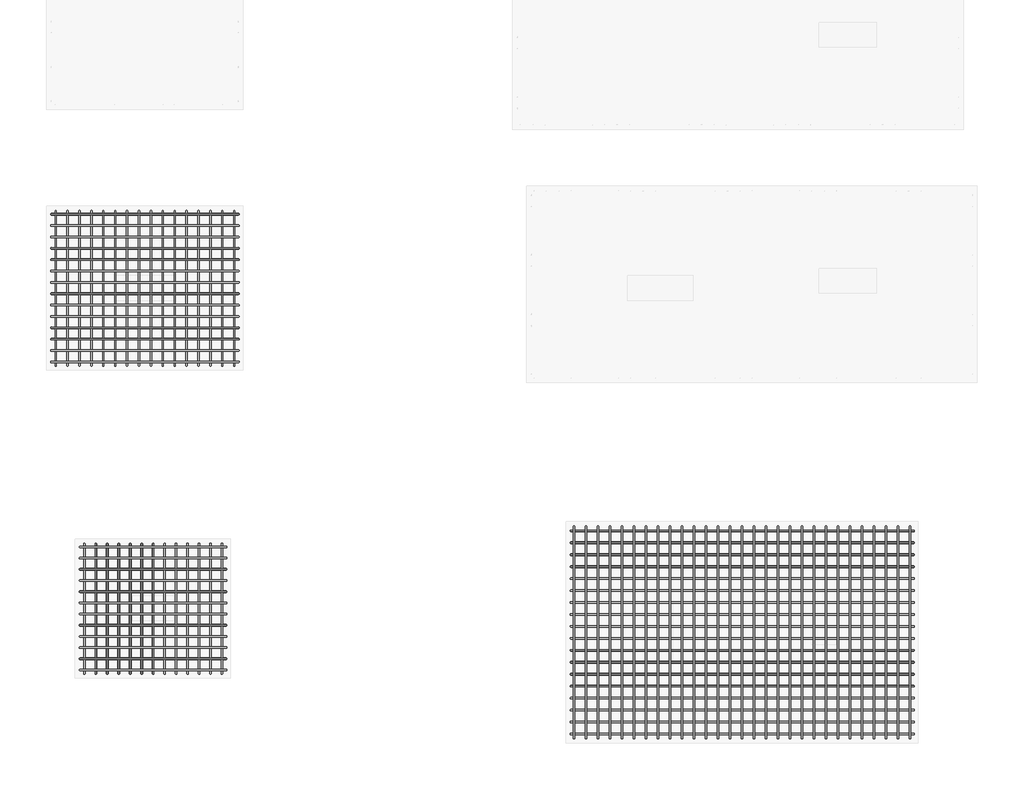
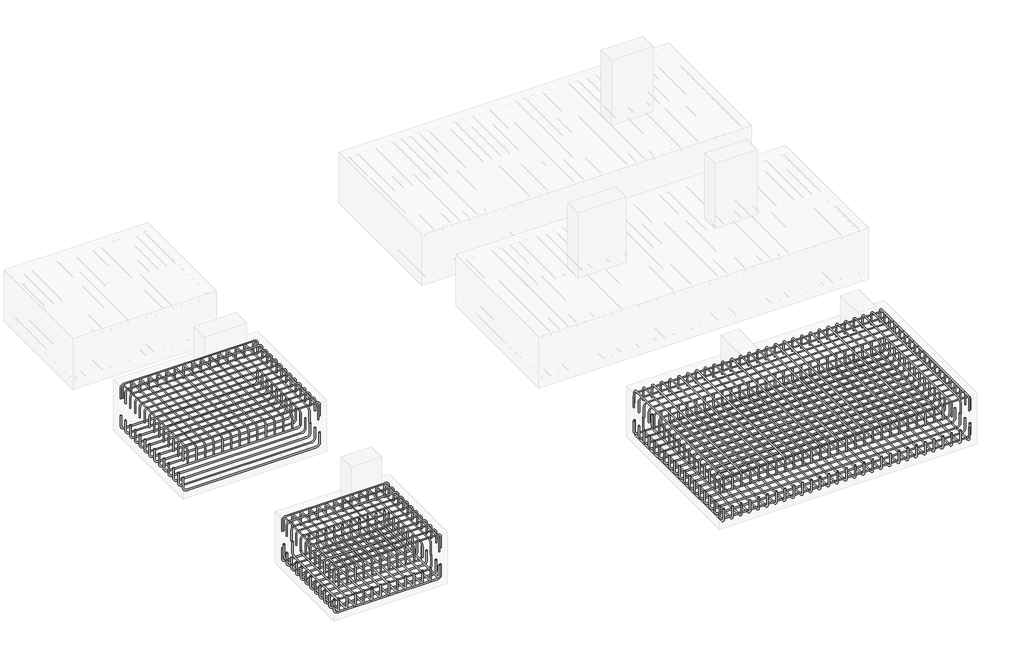
# One storey, part 3 of 21: 11 reinforcing bars.
"""IFC4 building model written with IfcOpenShell, lengths in millimetres."""

from ifc_helpers import new_model, si_unit, point, frame, origin, place, context, project, spatial, polyline, circle_curve, trimmed, segment, composite_curve, source, transform, mapped, element, save
from ifc_brep_helpers import swept_disk

model = new_model("IFC4")

# Units and contexts
model_context = context("Model", 3, world=origin())
ifc_project = project(units=[si_unit("LENGTHUNIT", "METRE", prefix="MILLI")], contexts=[model_context])

# Site, building, storey
site = spatial("IfcSite", under=ifc_project)
building = spatial("IfcBuilding", under=site)
storey = spatial("IfcBuildingStorey", under=building, Elevation=-1100.0)

# Reinforcing bars
placement = place(None, origin())
reinforcing_bar_shape = source(origin(), model_context, "Body", "SolidModel", [
    swept_disk(composite_curve([segment(polyline([(-23061.1351198, -6642.0783425, -1700.0), (-23061.1351198, -6642.0783425, -1882.5)]), True, "CONTINUOUS"), segment(trimmed(circle_curve(frame((-23118.6351198, -6642.0783425, -1882.5), z_axis=(0.0, 1.0, 0.0), x_axis=(57.5, 0.0, 0.0)), 57.5), [point((-23061.1351198, -6642.0783425, -1882.5))], [point((-23118.6351198, -6642.0783425, -1940.0))], True, "CARTESIAN"), True, "CONTINUOUS"), segment(polyline([(-23118.6351198, -6642.0783425, -1940.0), (-25283.6351198, -6642.0783425, -1940.0)]), True, "CONTINUOUS"), segment(trimmed(circle_curve(frame((-25283.6351198, -6642.0783425, -1882.5), z_axis=(0.0, 1.0, 0.0), x_axis=(0.0, 0.0, -57.5)), 57.5), [point((-25283.6351198, -6642.0783425, -1940.0))], [point((-25341.1351198, -6642.0783425, -1882.5))], True, "CARTESIAN"), True, "CONTINUOUS"), segment(polyline([(-25341.1351198, -6642.0783425, -1882.5), (-25341.1351198, -6642.0783425, -1700.0)]), True, "CONTINUOUS")], self_intersect=False), 10.0),
])
element("IfcReinforcingBar", 1, at=placement, inside=storey, context=model_context, shape_type="MappedRepresentation", body=[
    mapped(reinforcing_bar_shape, transform((0.0, 0.0, 0.0), x_axis=(1.0, 0.0, 0.0), y_axis=(0.0, 1.0, 0.0), z_axis=(0.0, 0.0, 1.0))),
    mapped(reinforcing_bar_shape, transform((0.0, -138.5928916, 0.0), x_axis=(1.0, 0.0, 0.0), y_axis=(0.0, 1.0, 0.0), z_axis=(0.0, 0.0, 1.0))),
    mapped(reinforcing_bar_shape, transform((0.0, -277.1857833, 0.0), x_axis=(1.0, 0.0, 0.0), y_axis=(0.0, 1.0, 0.0), z_axis=(0.0, 0.0, 1.0))),
    mapped(reinforcing_bar_shape, transform((0.0, -415.7786749, 0.0), x_axis=(1.0, 0.0, 0.0), y_axis=(0.0, 1.0, 0.0), z_axis=(0.0, 0.0, 1.0))),
    mapped(reinforcing_bar_shape, transform((0.0, -554.3715666, 0.0), x_axis=(1.0, 0.0, 0.0), y_axis=(0.0, 1.0, 0.0), z_axis=(0.0, 0.0, 1.0))),
    mapped(reinforcing_bar_shape, transform((0.0, -692.9644582, 0.0), x_axis=(1.0, 0.0, 0.0), y_axis=(0.0, 1.0, 0.0), z_axis=(0.0, 0.0, 1.0))),
    mapped(reinforcing_bar_shape, transform((0.0, -831.5573499, 0.0), x_axis=(1.0, 0.0, 0.0), y_axis=(0.0, 1.0, 0.0), z_axis=(0.0, 0.0, 1.0))),
    mapped(reinforcing_bar_shape, transform((0.0, -970.1502415, 0.0), x_axis=(1.0, 0.0, 0.0), y_axis=(0.0, 1.0, 0.0), z_axis=(0.0, 0.0, 1.0))),
    mapped(reinforcing_bar_shape, transform((0.0, -1108.7431331, 0.0), x_axis=(1.0, 0.0, 0.0), y_axis=(0.0, 1.0, 0.0), z_axis=(0.0, 0.0, 1.0))),
    mapped(reinforcing_bar_shape, transform((0.0, -1247.3360248, 0.0), x_axis=(1.0, 0.0, 0.0), y_axis=(0.0, 1.0, 0.0), z_axis=(0.0, 0.0, 1.0))),
    mapped(reinforcing_bar_shape, transform((0.0, -1385.9289164, 0.0), x_axis=(1.0, 0.0, 0.0), y_axis=(0.0, 1.0, 0.0), z_axis=(0.0, 0.0, 1.0))),
    mapped(reinforcing_bar_shape, transform((0.0, -1524.5218081, 0.0), x_axis=(1.0, 0.0, 0.0), y_axis=(0.0, 1.0, 0.0), z_axis=(0.0, 0.0, 1.0))),
    mapped(reinforcing_bar_shape, transform((0.0, -1663.1146997, 0.0), x_axis=(1.0, 0.0, 0.0), y_axis=(0.0, 1.0, 0.0), z_axis=(0.0, 0.0, 1.0))),
    mapped(reinforcing_bar_shape, transform((0.0, -1801.7075913, 0.0), x_axis=(1.0, 0.0, 0.0), y_axis=(0.0, 1.0, 0.0), z_axis=(0.0, 0.0, 1.0))),
])
reinforcing_bar_2_shape = source(origin(), model_context, "Body", "SolidModel", [
    swept_disk(composite_curve([segment(polyline([(-25343.1851198, -6642.0783425, -1400.0), (-25343.1851198, -6642.0783425, -1213.4)]), True, "CONTINUOUS"), segment(trimmed(circle_curve(frame((-25287.7351198, -6642.0783425, -1213.4), z_axis=(0.0, 1.0, 0.0), x_axis=(-55.45000000000073, 0.0, 0.0)), 55.45), [point((-25343.1851198, -6642.0783425, -1213.4))], [point((-25287.7351198, -6642.0783425, -1157.95))], True, "CARTESIAN"), True, "CONTINUOUS"), segment(polyline([(-25287.7351198, -6642.0783425, -1157.95), (-23114.5351198, -6642.0783425, -1157.95)]), True, "CONTINUOUS"), segment(trimmed(circle_curve(frame((-23114.5351198, -6642.0783425, -1213.4), z_axis=(0.0, 1.0, 0.0), x_axis=(0.0, 0.0, 55.450000000000045)), 55.45), [point((-23114.5351198, -6642.0783425, -1157.95))], [point((-23059.0851198, -6642.0783425, -1213.4))], True, "CARTESIAN"), True, "CONTINUOUS"), segment(polyline([(-23059.0851198, -6642.0783425, -1213.4), (-23059.0851198, -6642.0783425, -1400.0)]), True, "CONTINUOUS")], self_intersect=False), 7.95),
])
element("IfcReinforcingBar", 2, at=placement, inside=storey, context=model_context, shape_type="MappedRepresentation", body=[
    mapped(reinforcing_bar_2_shape, transform((0.0, 0.0, 0.0), x_axis=(1.0, 0.0, 0.0), y_axis=(0.0, 1.0, 0.0), z_axis=(0.0, 0.0, 1.0))),
    mapped(reinforcing_bar_2_shape, transform((0.0, -138.5928916, 0.0), x_axis=(1.0, 0.0, 0.0), y_axis=(0.0, 1.0, 0.0), z_axis=(0.0, 0.0, 1.0))),
    mapped(reinforcing_bar_2_shape, transform((0.0, -277.1857833, 0.0), x_axis=(1.0, 0.0, 0.0), y_axis=(0.0, 1.0, 0.0), z_axis=(0.0, 0.0, 1.0))),
    mapped(reinforcing_bar_2_shape, transform((0.0, -415.7786749, 0.0), x_axis=(1.0, 0.0, 0.0), y_axis=(0.0, 1.0, 0.0), z_axis=(0.0, 0.0, 1.0))),
    mapped(reinforcing_bar_2_shape, transform((0.0, -554.3715666, 0.0), x_axis=(1.0, 0.0, 0.0), y_axis=(0.0, 1.0, 0.0), z_axis=(0.0, 0.0, 1.0))),
    mapped(reinforcing_bar_2_shape, transform((0.0, -692.9644582, 0.0), x_axis=(1.0, 0.0, 0.0), y_axis=(0.0, 1.0, 0.0), z_axis=(0.0, 0.0, 1.0))),
    mapped(reinforcing_bar_2_shape, transform((0.0, -831.5573499, 0.0), x_axis=(1.0, 0.0, 0.0), y_axis=(0.0, 1.0, 0.0), z_axis=(0.0, 0.0, 1.0))),
    mapped(reinforcing_bar_2_shape, transform((0.0, -970.1502415, 0.0), x_axis=(1.0, 0.0, 0.0), y_axis=(0.0, 1.0, 0.0), z_axis=(0.0, 0.0, 1.0))),
    mapped(reinforcing_bar_2_shape, transform((0.0, -1108.7431331, 0.0), x_axis=(1.0, 0.0, 0.0), y_axis=(0.0, 1.0, 0.0), z_axis=(0.0, 0.0, 1.0))),
    mapped(reinforcing_bar_2_shape, transform((0.0, -1247.3360248, 0.0), x_axis=(1.0, 0.0, 0.0), y_axis=(0.0, 1.0, 0.0), z_axis=(0.0, 0.0, 1.0))),
    mapped(reinforcing_bar_2_shape, transform((0.0, -1385.9289164, 0.0), x_axis=(1.0, 0.0, 0.0), y_axis=(0.0, 1.0, 0.0), z_axis=(0.0, 0.0, 1.0))),
    mapped(reinforcing_bar_2_shape, transform((0.0, -1524.5218081, 0.0), x_axis=(1.0, 0.0, 0.0), y_axis=(0.0, 1.0, 0.0), z_axis=(0.0, 0.0, 1.0))),
    mapped(reinforcing_bar_2_shape, transform((0.0, -1663.1146997, 0.0), x_axis=(1.0, 0.0, 0.0), y_axis=(0.0, 1.0, 0.0), z_axis=(0.0, 0.0, 1.0))),
    mapped(reinforcing_bar_2_shape, transform((0.0, -1801.7075913, 0.0), x_axis=(1.0, 0.0, 0.0), y_axis=(0.0, 1.0, 0.0), z_axis=(0.0, 0.0, 1.0))),
])
reinforcing_bar_3_shape = source(origin(), model_context, "Body", "SolidModel", [
    swept_disk(composite_curve([segment(polyline([(-23110.9192838, -6603.7795712, -1428.1111113), (-23110.9192838, -6603.7795712, -1241.5111113)]), True, "CONTINUOUS"), segment(trimmed(circle_curve(frame((-23110.9192838, -6659.2295712, -1241.5111113), z_axis=(1.0, 0.0, 0.0), x_axis=(0.0, 55.44999999999982, 0.0)), 55.45), [point((-23110.9192838, -6603.7795712, -1241.5111113))], [point((-23110.9192838, -6659.2295712, -1186.0611113))], True, "CARTESIAN"), True, "CONTINUOUS"), segment(polyline([(-23110.9192838, -6659.2295712, -1186.0611113), (-23110.9192838, -8432.4295712, -1186.0611113)]), True, "CONTINUOUS"), segment(trimmed(circle_curve(frame((-23110.9192838, -8432.4295712, -1241.5111113), z_axis=(1.0, 0.0, 0.0), x_axis=(0.0, 0.0, 55.450000000000045)), 55.45), [point((-23110.9192838, -8432.4295712, -1186.0611113))], [point((-23110.9192838, -8487.8795712, -1241.5111113))], True, "CARTESIAN"), True, "CONTINUOUS"), segment(polyline([(-23110.9192838, -8487.8795712, -1241.5111113), (-23110.9192838, -8487.8795712, -1428.1111113)]), True, "CONTINUOUS")], self_intersect=False), 7.95),
])
element("IfcReinforcingBar", 3, at=placement, inside=storey, context=model_context, shape_type="MappedRepresentation", body=[
    mapped(reinforcing_bar_3_shape, transform((0.0, 0.0, 0.0), x_axis=(1.0, 0.0, 0.0), y_axis=(0.0, 1.0, 0.0), z_axis=(0.0, 0.0, 1.0))),
    mapped(reinforcing_bar_3_shape, transform((-145.2528929, 0.0, 0.0), x_axis=(1.0, 0.0, 0.0), y_axis=(0.0, 1.0, 0.0), z_axis=(0.0, 0.0, 1.0))),
    mapped(reinforcing_bar_3_shape, transform((-290.5057858, 0.0, 0.0), x_axis=(1.0, 0.0, 0.0), y_axis=(0.0, 1.0, 0.0), z_axis=(0.0, 0.0, 1.0))),
    mapped(reinforcing_bar_3_shape, transform((-435.7586787, 0.0, 0.0), x_axis=(1.0, 0.0, 0.0), y_axis=(0.0, 1.0, 0.0), z_axis=(0.0, 0.0, 1.0))),
    mapped(reinforcing_bar_3_shape, transform((-581.0115716, 0.0, 0.0), x_axis=(1.0, 0.0, 0.0), y_axis=(0.0, 1.0, 0.0), z_axis=(0.0, 0.0, 1.0))),
    mapped(reinforcing_bar_3_shape, transform((-726.2644645, 0.0, 0.0), x_axis=(1.0, 0.0, 0.0), y_axis=(0.0, 1.0, 0.0), z_axis=(0.0, 0.0, 1.0))),
    mapped(reinforcing_bar_3_shape, transform((-871.5173574, 0.0, 0.0), x_axis=(1.0, 0.0, 0.0), y_axis=(0.0, 1.0, 0.0), z_axis=(0.0, 0.0, 1.0))),
    mapped(reinforcing_bar_3_shape, transform((-1016.7702503, 0.0, 0.0), x_axis=(1.0, 0.0, 0.0), y_axis=(0.0, 1.0, 0.0), z_axis=(0.0, 0.0, 1.0))),
    mapped(reinforcing_bar_3_shape, transform((-1162.0231432, 0.0, 0.0), x_axis=(1.0, 0.0, 0.0), y_axis=(0.0, 1.0, 0.0), z_axis=(0.0, 0.0, 1.0))),
    mapped(reinforcing_bar_3_shape, transform((-1307.276036, 0.0, 0.0), x_axis=(1.0, 0.0, 0.0), y_axis=(0.0, 1.0, 0.0), z_axis=(0.0, 0.0, 1.0))),
    mapped(reinforcing_bar_3_shape, transform((-1452.5289289, 0.0, 0.0), x_axis=(1.0, 0.0, 0.0), y_axis=(0.0, 1.0, 0.0), z_axis=(0.0, 0.0, 1.0))),
    mapped(reinforcing_bar_3_shape, transform((-1597.7818218, 0.0, 0.0), x_axis=(1.0, 0.0, 0.0), y_axis=(0.0, 1.0, 0.0), z_axis=(0.0, 0.0, 1.0))),
    mapped(reinforcing_bar_3_shape, transform((-1743.0347147, 0.0, 0.0), x_axis=(1.0, 0.0, 0.0), y_axis=(0.0, 1.0, 0.0), z_axis=(0.0, 0.0, 1.0))),
    mapped(reinforcing_bar_3_shape, transform((-1888.2876076, 0.0, 0.0), x_axis=(1.0, 0.0, 0.0), y_axis=(0.0, 1.0, 0.0), z_axis=(0.0, 0.0, 1.0))),
    mapped(reinforcing_bar_3_shape, transform((-2033.5405005, 0.0, 0.0), x_axis=(1.0, 0.0, 0.0), y_axis=(0.0, 1.0, 0.0), z_axis=(0.0, 0.0, 1.0))),
    mapped(reinforcing_bar_3_shape, transform((-2178.7933934, 0.0, 0.0), x_axis=(1.0, 0.0, 0.0), y_axis=(0.0, 1.0, 0.0), z_axis=(0.0, 0.0, 1.0))),
])
reinforcing_bar_4_shape = source(origin(), model_context, "Body", "SolidModel", [
    swept_disk(composite_curve([segment(polyline([(-23210.8326863, -10702.0783425, -1700.0), (-23210.8326863, -10702.0783425, -1882.5)]), True, "CONTINUOUS"), segment(trimmed(circle_curve(frame((-23268.3326863, -10702.0783425, -1882.5), z_axis=(0.0, 1.0, 0.0), x_axis=(57.5, 0.0, 0.0)), 57.5), [point((-23210.8326863, -10702.0783425, -1882.5))], [point((-23268.3326863, -10702.0783425, -1940.0))], True, "CARTESIAN"), True, "CONTINUOUS"), segment(polyline([(-23268.3326863, -10702.0783425, -1940.0), (-24933.3326863, -10702.0783425, -1940.0)]), True, "CONTINUOUS"), segment(trimmed(circle_curve(frame((-24933.3326863, -10702.0783425, -1882.5), z_axis=(0.0, 1.0, 0.0), x_axis=(0.0, 0.0, -57.5)), 57.5), [point((-24933.3326863, -10702.0783425, -1940.0))], [point((-24990.8326863, -10702.0783425, -1882.5))], True, "CARTESIAN"), True, "CONTINUOUS"), segment(polyline([(-24990.8326863, -10702.0783425, -1882.5), (-24990.8326863, -10702.0783425, -1700.0)]), True, "CONTINUOUS")], self_intersect=False), 10.0),
])
element("IfcReinforcingBar", 4, at=placement, inside=storey, context=model_context, shape_type="MappedRepresentation", body=[
    mapped(reinforcing_bar_4_shape, transform((0.0, 0.0, 0.0), x_axis=(1.0, 0.0, 0.0), y_axis=(0.0, 1.0, 0.0), z_axis=(0.0, 0.0, 1.0))),
    mapped(reinforcing_bar_4_shape, transform((0.0, -136.5188719, 0.0), x_axis=(1.0, 0.0, 0.0), y_axis=(0.0, 1.0, 0.0), z_axis=(0.0, 0.0, 1.0))),
    mapped(reinforcing_bar_4_shape, transform((0.0, -273.0377439, 0.0), x_axis=(1.0, 0.0, 0.0), y_axis=(0.0, 1.0, 0.0), z_axis=(0.0, 0.0, 1.0))),
    mapped(reinforcing_bar_4_shape, transform((0.0, -409.5566158, 0.0), x_axis=(1.0, 0.0, 0.0), y_axis=(0.0, 1.0, 0.0), z_axis=(0.0, 0.0, 1.0))),
    mapped(reinforcing_bar_4_shape, transform((0.0, -546.0754878, 0.0), x_axis=(1.0, 0.0, 0.0), y_axis=(0.0, 1.0, 0.0), z_axis=(0.0, 0.0, 1.0))),
    mapped(reinforcing_bar_4_shape, transform((0.0, -682.5943597, 0.0), x_axis=(1.0, 0.0, 0.0), y_axis=(0.0, 1.0, 0.0), z_axis=(0.0, 0.0, 1.0))),
    mapped(reinforcing_bar_4_shape, transform((0.0, -819.1132316, 0.0), x_axis=(1.0, 0.0, 0.0), y_axis=(0.0, 1.0, 0.0), z_axis=(0.0, 0.0, 1.0))),
    mapped(reinforcing_bar_4_shape, transform((0.0, -955.6321036, 0.0), x_axis=(1.0, 0.0, 0.0), y_axis=(0.0, 1.0, 0.0), z_axis=(0.0, 0.0, 1.0))),
    mapped(reinforcing_bar_4_shape, transform((0.0, -1092.1509755, 0.0), x_axis=(1.0, 0.0, 0.0), y_axis=(0.0, 1.0, 0.0), z_axis=(0.0, 0.0, 1.0))),
    mapped(reinforcing_bar_4_shape, transform((0.0, -1228.6698475, 0.0), x_axis=(1.0, 0.0, 0.0), y_axis=(0.0, 1.0, 0.0), z_axis=(0.0, 0.0, 1.0))),
    mapped(reinforcing_bar_4_shape, transform((0.0, -1365.1887194, 0.0), x_axis=(1.0, 0.0, 0.0), y_axis=(0.0, 1.0, 0.0), z_axis=(0.0, 0.0, 1.0))),
    mapped(reinforcing_bar_4_shape, transform((0.0, -1501.7075913, 0.0), x_axis=(1.0, 0.0, 0.0), y_axis=(0.0, 1.0, 0.0), z_axis=(0.0, 0.0, 1.0))),
])
reinforcing_bar_5_shape = source(origin(), model_context, "Body", "SolidModel", [
    swept_disk(composite_curve([segment(polyline([(-24992.8826863, -10702.0783425, -1400.0), (-24992.8826863, -10702.0783425, -1213.4)]), True, "CONTINUOUS"), segment(trimmed(circle_curve(frame((-24937.4326863, -10702.0783425, -1213.4), z_axis=(0.0, 1.0, 0.0), x_axis=(-55.45000000000073, 0.0, 0.0)), 55.45), [point((-24992.8826863, -10702.0783425, -1213.4))], [point((-24937.4326863, -10702.0783425, -1157.95))], True, "CARTESIAN"), True, "CONTINUOUS"), segment(polyline([(-24937.4326863, -10702.0783425, -1157.95), (-23264.2326863, -10702.0783425, -1157.95)]), True, "CONTINUOUS"), segment(trimmed(circle_curve(frame((-23264.2326863, -10702.0783425, -1213.4), z_axis=(0.0, 1.0, 0.0), x_axis=(0.0, 0.0, 55.450000000000045)), 55.45), [point((-23264.2326863, -10702.0783425, -1157.95))], [point((-23208.7826863, -10702.0783425, -1213.4))], True, "CARTESIAN"), True, "CONTINUOUS"), segment(polyline([(-23208.7826863, -10702.0783425, -1213.4), (-23208.7826863, -10702.0783425, -1400.0)]), True, "CONTINUOUS")], self_intersect=False), 7.95),
])
element("IfcReinforcingBar", 5, at=placement, inside=storey, context=model_context, shape_type="MappedRepresentation", body=[
    mapped(reinforcing_bar_5_shape, transform((0.0, 0.0, 0.0), x_axis=(1.0, 0.0, 0.0), y_axis=(0.0, 1.0, 0.0), z_axis=(0.0, 0.0, 1.0))),
    mapped(reinforcing_bar_5_shape, transform((0.0, -136.5188719, 0.0), x_axis=(1.0, 0.0, 0.0), y_axis=(0.0, 1.0, 0.0), z_axis=(0.0, 0.0, 1.0))),
    mapped(reinforcing_bar_5_shape, transform((0.0, -273.0377439, 0.0), x_axis=(1.0, 0.0, 0.0), y_axis=(0.0, 1.0, 0.0), z_axis=(0.0, 0.0, 1.0))),
    mapped(reinforcing_bar_5_shape, transform((0.0, -409.5566158, 0.0), x_axis=(1.0, 0.0, 0.0), y_axis=(0.0, 1.0, 0.0), z_axis=(0.0, 0.0, 1.0))),
    mapped(reinforcing_bar_5_shape, transform((0.0, -546.0754878, 0.0), x_axis=(1.0, 0.0, 0.0), y_axis=(0.0, 1.0, 0.0), z_axis=(0.0, 0.0, 1.0))),
    mapped(reinforcing_bar_5_shape, transform((0.0, -682.5943597, 0.0), x_axis=(1.0, 0.0, 0.0), y_axis=(0.0, 1.0, 0.0), z_axis=(0.0, 0.0, 1.0))),
    mapped(reinforcing_bar_5_shape, transform((0.0, -819.1132316, 0.0), x_axis=(1.0, 0.0, 0.0), y_axis=(0.0, 1.0, 0.0), z_axis=(0.0, 0.0, 1.0))),
    mapped(reinforcing_bar_5_shape, transform((0.0, -955.6321036, 0.0), x_axis=(1.0, 0.0, 0.0), y_axis=(0.0, 1.0, 0.0), z_axis=(0.0, 0.0, 1.0))),
    mapped(reinforcing_bar_5_shape, transform((0.0, -1092.1509755, 0.0), x_axis=(1.0, 0.0, 0.0), y_axis=(0.0, 1.0, 0.0), z_axis=(0.0, 0.0, 1.0))),
    mapped(reinforcing_bar_5_shape, transform((0.0, -1228.6698475, 0.0), x_axis=(1.0, 0.0, 0.0), y_axis=(0.0, 1.0, 0.0), z_axis=(0.0, 0.0, 1.0))),
    mapped(reinforcing_bar_5_shape, transform((0.0, -1365.1887194, 0.0), x_axis=(1.0, 0.0, 0.0), y_axis=(0.0, 1.0, 0.0), z_axis=(0.0, 0.0, 1.0))),
    mapped(reinforcing_bar_5_shape, transform((0.0, -1501.7075913, 0.0), x_axis=(1.0, 0.0, 0.0), y_axis=(0.0, 1.0, 0.0), z_axis=(0.0, 0.0, 1.0))),
])
reinforcing_bar_6_shape = source(origin(), model_context, "Body", "SolidModel", [
    swept_disk(composite_curve([segment(polyline([(-23260.6168504, -10663.7795712, -1428.1111113), (-23260.6168504, -10663.7795712, -1241.5111113)]), True, "CONTINUOUS"), segment(trimmed(circle_curve(frame((-23260.6168504, -10719.2295712, -1241.5111113), z_axis=(1.0, 0.0, 0.0), x_axis=(0.0, 55.44999999999891, 0.0)), 55.45), [point((-23260.6168504, -10663.7795712, -1241.5111113))], [point((-23260.6168504, -10719.2295712, -1186.0611113))], True, "CARTESIAN"), True, "CONTINUOUS"), segment(polyline([(-23260.6168504, -10719.2295712, -1186.0611113), (-23260.6168504, -12192.4295712, -1186.0611113)]), True, "CONTINUOUS"), segment(trimmed(circle_curve(frame((-23260.6168504, -12192.4295712, -1241.5111113), z_axis=(1.0, 0.0, 0.0), x_axis=(0.0, 0.0, 55.450000000000045)), 55.45), [point((-23260.6168504, -12192.4295712, -1186.0611113))], [point((-23260.6168504, -12247.8795712, -1241.5111113))], True, "CARTESIAN"), True, "CONTINUOUS"), segment(polyline([(-23260.6168504, -12247.8795712, -1241.5111113), (-23260.6168504, -12247.8795712, -1428.1111113)]), True, "CONTINUOUS")], self_intersect=False), 7.95),
])
element("IfcReinforcingBar", 6, at=placement, inside=storey, context=model_context, shape_type="MappedRepresentation", body=[
    mapped(reinforcing_bar_6_shape, transform((0.0, 0.0, 0.0), x_axis=(1.0, 0.0, 0.0), y_axis=(0.0, 1.0, 0.0), z_axis=(0.0, 0.0, 1.0))),
    mapped(reinforcing_bar_6_shape, transform((-139.8994495, 0.0, 0.0), x_axis=(1.0, 0.0, 0.0), y_axis=(0.0, 1.0, 0.0), z_axis=(0.0, 0.0, 1.0))),
    mapped(reinforcing_bar_6_shape, transform((-279.7988989, 0.0, 0.0), x_axis=(1.0, 0.0, 0.0), y_axis=(0.0, 1.0, 0.0), z_axis=(0.0, 0.0, 1.0))),
    mapped(reinforcing_bar_6_shape, transform((-419.6983484, 0.0, 0.0), x_axis=(1.0, 0.0, 0.0), y_axis=(0.0, 1.0, 0.0), z_axis=(0.0, 0.0, 1.0))),
    mapped(reinforcing_bar_6_shape, transform((-559.5977978, 0.0, 0.0), x_axis=(1.0, 0.0, 0.0), y_axis=(0.0, 1.0, 0.0), z_axis=(0.0, 0.0, 1.0))),
    mapped(reinforcing_bar_6_shape, transform((-699.4972473, 0.0, 0.0), x_axis=(1.0, 0.0, 0.0), y_axis=(0.0, 1.0, 0.0), z_axis=(0.0, 0.0, 1.0))),
    mapped(reinforcing_bar_6_shape, transform((-839.3966967, 0.0, 0.0), x_axis=(1.0, 0.0, 0.0), y_axis=(0.0, 1.0, 0.0), z_axis=(0.0, 0.0, 1.0))),
    mapped(reinforcing_bar_6_shape, transform((-979.2961462, 0.0, 0.0), x_axis=(1.0, 0.0, 0.0), y_axis=(0.0, 1.0, 0.0), z_axis=(0.0, 0.0, 1.0))),
    mapped(reinforcing_bar_6_shape, transform((-1119.1955956, 0.0, 0.0), x_axis=(1.0, 0.0, 0.0), y_axis=(0.0, 1.0, 0.0), z_axis=(0.0, 0.0, 1.0))),
    mapped(reinforcing_bar_6_shape, transform((-1259.0950451, 0.0, 0.0), x_axis=(1.0, 0.0, 0.0), y_axis=(0.0, 1.0, 0.0), z_axis=(0.0, 0.0, 1.0))),
    mapped(reinforcing_bar_6_shape, transform((-1398.9944945, 0.0, 0.0), x_axis=(1.0, 0.0, 0.0), y_axis=(0.0, 1.0, 0.0), z_axis=(0.0, 0.0, 1.0))),
    mapped(reinforcing_bar_6_shape, transform((-1538.893944, 0.0, 0.0), x_axis=(1.0, 0.0, 0.0), y_axis=(0.0, 1.0, 0.0), z_axis=(0.0, 0.0, 1.0))),
    mapped(reinforcing_bar_6_shape, transform((-1678.7933934, 0.0, 0.0), x_axis=(1.0, 0.0, 0.0), y_axis=(0.0, 1.0, 0.0), z_axis=(0.0, 0.0, 1.0))),
])
reinforcing_bar_7_shape = source(origin(), model_context, "Body", "SolidModel", [
    swept_disk(composite_curve([segment(polyline([(-24939.4102438, -10665.8295712, -1669.8442859), (-24939.4102438, -10665.8295712, -1852.3442859)]), True, "CONTINUOUS"), segment(trimmed(circle_curve(frame((-24939.4102438, -10723.3295712, -1852.3442859), z_axis=(-1.0, 0.0, 0.0), x_axis=(0.0, 57.5, 0.0)), 57.5), [point((-24939.4102438, -10665.8295712, -1852.3442859))], [point((-24939.4102438, -10723.3295712, -1909.8442859))], True, "CARTESIAN"), True, "CONTINUOUS"), segment(polyline([(-24939.4102438, -10723.3295712, -1909.8442859), (-24939.4102438, -12188.3295712, -1909.8442859)]), True, "CONTINUOUS"), segment(trimmed(circle_curve(frame((-24939.4102438, -12188.3295712, -1852.3442859), z_axis=(-1.0, 0.0, 0.0), x_axis=(0.0, 0.0, -57.5)), 57.5), [point((-24939.4102438, -12188.3295712, -1909.8442859))], [point((-24939.4102438, -12245.8295712, -1852.3442859))], True, "CARTESIAN"), True, "CONTINUOUS"), segment(polyline([(-24939.4102438, -12245.8295712, -1852.3442859), (-24939.4102438, -12245.8295712, -1669.8442859)]), True, "CONTINUOUS")], self_intersect=False), 10.0),
])
element("IfcReinforcingBar", 7, at=placement, inside=storey, context=model_context, shape_type="MappedRepresentation", body=[
    mapped(reinforcing_bar_7_shape, transform((0.0, 0.0, 0.0), x_axis=(1.0, 0.0, 0.0), y_axis=(0.0, 1.0, 0.0), z_axis=(0.0, 0.0, 1.0))),
    mapped(reinforcing_bar_7_shape, transform((139.8994495, 0.0, 0.0), x_axis=(1.0, 0.0, 0.0), y_axis=(0.0, 1.0, 0.0), z_axis=(0.0, 0.0, 1.0))),
    mapped(reinforcing_bar_7_shape, transform((279.7988989, 0.0, 0.0), x_axis=(1.0, 0.0, 0.0), y_axis=(0.0, 1.0, 0.0), z_axis=(0.0, 0.0, 1.0))),
    mapped(reinforcing_bar_7_shape, transform((419.6983484, 0.0, 0.0), x_axis=(1.0, 0.0, 0.0), y_axis=(0.0, 1.0, 0.0), z_axis=(0.0, 0.0, 1.0))),
    mapped(reinforcing_bar_7_shape, transform((559.5977978, 0.0, 0.0), x_axis=(1.0, 0.0, 0.0), y_axis=(0.0, 1.0, 0.0), z_axis=(0.0, 0.0, 1.0))),
    mapped(reinforcing_bar_7_shape, transform((699.4972473, 0.0, 0.0), x_axis=(1.0, 0.0, 0.0), y_axis=(0.0, 1.0, 0.0), z_axis=(0.0, 0.0, 1.0))),
    mapped(reinforcing_bar_7_shape, transform((839.3966967, 0.0, 0.0), x_axis=(1.0, 0.0, 0.0), y_axis=(0.0, 1.0, 0.0), z_axis=(0.0, 0.0, 1.0))),
    mapped(reinforcing_bar_7_shape, transform((979.2961462, 0.0, 0.0), x_axis=(1.0, 0.0, 0.0), y_axis=(0.0, 1.0, 0.0), z_axis=(0.0, 0.0, 1.0))),
    mapped(reinforcing_bar_7_shape, transform((1119.1955956, 0.0, 0.0), x_axis=(1.0, 0.0, 0.0), y_axis=(0.0, 1.0, 0.0), z_axis=(0.0, 0.0, 1.0))),
    mapped(reinforcing_bar_7_shape, transform((1259.0950451, 0.0, 0.0), x_axis=(1.0, 0.0, 0.0), y_axis=(0.0, 1.0, 0.0), z_axis=(0.0, 0.0, 1.0))),
    mapped(reinforcing_bar_7_shape, transform((1398.9944945, 0.0, 0.0), x_axis=(1.0, 0.0, 0.0), y_axis=(0.0, 1.0, 0.0), z_axis=(0.0, 0.0, 1.0))),
    mapped(reinforcing_bar_7_shape, transform((1538.893944, 0.0, 0.0), x_axis=(1.0, 0.0, 0.0), y_axis=(0.0, 1.0, 0.0), z_axis=(0.0, 0.0, 1.0))),
    mapped(reinforcing_bar_7_shape, transform((1678.7933934, 0.0, 0.0), x_axis=(1.0, 0.0, 0.0), y_axis=(0.0, 1.0, 0.0), z_axis=(0.0, 0.0, 1.0))),
])
reinforcing_bar_8_shape = source(origin(), model_context, "Body", "SolidModel", [
    swept_disk(composite_curve([segment(polyline([(-18964.5839151, -10455.8295712, -1700.0), (-18964.5839151, -10455.8295712, -1882.5)]), True, "CONTINUOUS"), segment(trimmed(circle_curve(frame((-18964.5839151, -10513.3295712, -1882.5), z_axis=(-1.0, 0.0, 0.0), x_axis=(0.0, 57.5, 0.0)), 57.5), [point((-18964.5839151, -10455.8295712, -1882.5))], [point((-18964.5839151, -10513.3295712, -1940.0))], True, "CARTESIAN"), True, "CONTINUOUS"), segment(polyline([(-18964.5839151, -10513.3295712, -1940.0), (-18964.5839151, -12978.3295712, -1940.0)]), True, "CONTINUOUS"), segment(trimmed(circle_curve(frame((-18964.5839151, -12978.3295712, -1882.5), z_axis=(-1.0, 0.0, 0.0), x_axis=(0.0, 0.0, -57.5)), 57.5), [point((-18964.5839151, -12978.3295712, -1940.0))], [point((-18964.5839151, -13035.8295712, -1882.5))], True, "CARTESIAN"), True, "CONTINUOUS"), segment(polyline([(-18964.5839151, -13035.8295712, -1882.5), (-18964.5839151, -13035.8295712, -1700.0)]), True, "CONTINUOUS")], self_intersect=False), 10.0),
])
element("IfcReinforcingBar", 8, at=placement, inside=storey, context=model_context, shape_type="MappedRepresentation", body=[
    mapped(reinforcing_bar_8_shape, transform((0.0, 0.0, 0.0), x_axis=(1.0, 0.0, 0.0), y_axis=(0.0, 1.0, 0.0), z_axis=(0.0, 0.0, 1.0))),
    mapped(reinforcing_bar_8_shape, transform((146.4895568, 0.0, 0.0), x_axis=(1.0, 0.0, 0.0), y_axis=(0.0, 1.0, 0.0), z_axis=(0.0, 0.0, 1.0))),
    mapped(reinforcing_bar_8_shape, transform((292.9791137, 0.0, 0.0), x_axis=(1.0, 0.0, 0.0), y_axis=(0.0, 1.0, 0.0), z_axis=(0.0, 0.0, 1.0))),
    mapped(reinforcing_bar_8_shape, transform((439.4686705, 0.0, 0.0), x_axis=(1.0, 0.0, 0.0), y_axis=(0.0, 1.0, 0.0), z_axis=(0.0, 0.0, 1.0))),
    mapped(reinforcing_bar_8_shape, transform((585.9582273, 0.0, 0.0), x_axis=(1.0, 0.0, 0.0), y_axis=(0.0, 1.0, 0.0), z_axis=(0.0, 0.0, 1.0))),
    mapped(reinforcing_bar_8_shape, transform((732.4477842, 0.0, 0.0), x_axis=(1.0, 0.0, 0.0), y_axis=(0.0, 1.0, 0.0), z_axis=(0.0, 0.0, 1.0))),
    mapped(reinforcing_bar_8_shape, transform((878.937341, 0.0, 0.0), x_axis=(1.0, 0.0, 0.0), y_axis=(0.0, 1.0, 0.0), z_axis=(0.0, 0.0, 1.0))),
    mapped(reinforcing_bar_8_shape, transform((1025.4268978, 0.0, 0.0), x_axis=(1.0, 0.0, 0.0), y_axis=(0.0, 1.0, 0.0), z_axis=(0.0, 0.0, 1.0))),
    mapped(reinforcing_bar_8_shape, transform((1171.9164547, 0.0, 0.0), x_axis=(1.0, 0.0, 0.0), y_axis=(0.0, 1.0, 0.0), z_axis=(0.0, 0.0, 1.0))),
    mapped(reinforcing_bar_8_shape, transform((1318.4060115, 0.0, 0.0), x_axis=(1.0, 0.0, 0.0), y_axis=(0.0, 1.0, 0.0), z_axis=(0.0, 0.0, 1.0))),
    mapped(reinforcing_bar_8_shape, transform((1464.8955683, 0.0, 0.0), x_axis=(1.0, 0.0, 0.0), y_axis=(0.0, 1.0, 0.0), z_axis=(0.0, 0.0, 1.0))),
    mapped(reinforcing_bar_8_shape, transform((1611.3851252, 0.0, 0.0), x_axis=(1.0, 0.0, 0.0), y_axis=(0.0, 1.0, 0.0), z_axis=(0.0, 0.0, 1.0))),
    mapped(reinforcing_bar_8_shape, transform((1757.874682, 0.0, 0.0), x_axis=(1.0, 0.0, 0.0), y_axis=(0.0, 1.0, 0.0), z_axis=(0.0, 0.0, 1.0))),
    mapped(reinforcing_bar_8_shape, transform((1904.3642388, 0.0, 0.0), x_axis=(1.0, 0.0, 0.0), y_axis=(0.0, 1.0, 0.0), z_axis=(0.0, 0.0, 1.0))),
    mapped(reinforcing_bar_8_shape, transform((2050.8537957, 0.0, 0.0), x_axis=(1.0, 0.0, 0.0), y_axis=(0.0, 1.0, 0.0), z_axis=(0.0, 0.0, 1.0))),
    mapped(reinforcing_bar_8_shape, transform((2197.3433525, 0.0, 0.0), x_axis=(1.0, 0.0, 0.0), y_axis=(0.0, 1.0, 0.0), z_axis=(0.0, 0.0, 1.0))),
    mapped(reinforcing_bar_8_shape, transform((2343.8329093, 0.0, 0.0), x_axis=(1.0, 0.0, 0.0), y_axis=(0.0, 1.0, 0.0), z_axis=(0.0, 0.0, 1.0))),
    mapped(reinforcing_bar_8_shape, transform((2490.3224662, 0.0, 0.0), x_axis=(1.0, 0.0, 0.0), y_axis=(0.0, 1.0, 0.0), z_axis=(0.0, 0.0, 1.0))),
    mapped(reinforcing_bar_8_shape, transform((2636.812023, 0.0, 0.0), x_axis=(1.0, 0.0, 0.0), y_axis=(0.0, 1.0, 0.0), z_axis=(0.0, 0.0, 1.0))),
    mapped(reinforcing_bar_8_shape, transform((2783.3015798, 0.0, 0.0), x_axis=(1.0, 0.0, 0.0), y_axis=(0.0, 1.0, 0.0), z_axis=(0.0, 0.0, 1.0))),
    mapped(reinforcing_bar_8_shape, transform((2929.7911367, 0.0, 0.0), x_axis=(1.0, 0.0, 0.0), y_axis=(0.0, 1.0, 0.0), z_axis=(0.0, 0.0, 1.0))),
    mapped(reinforcing_bar_8_shape, transform((3076.2806935, 0.0, 0.0), x_axis=(1.0, 0.0, 0.0), y_axis=(0.0, 1.0, 0.0), z_axis=(0.0, 0.0, 1.0))),
    mapped(reinforcing_bar_8_shape, transform((3222.7702503, 0.0, 0.0), x_axis=(1.0, 0.0, 0.0), y_axis=(0.0, 1.0, 0.0), z_axis=(0.0, 0.0, 1.0))),
    mapped(reinforcing_bar_8_shape, transform((3369.2598072, 0.0, 0.0), x_axis=(1.0, 0.0, 0.0), y_axis=(0.0, 1.0, 0.0), z_axis=(0.0, 0.0, 1.0))),
    mapped(reinforcing_bar_8_shape, transform((3515.749364, 0.0, 0.0), x_axis=(1.0, 0.0, 0.0), y_axis=(0.0, 1.0, 0.0), z_axis=(0.0, 0.0, 1.0))),
    mapped(reinforcing_bar_8_shape, transform((3662.2389208, 0.0, 0.0), x_axis=(1.0, 0.0, 0.0), y_axis=(0.0, 1.0, 0.0), z_axis=(0.0, 0.0, 1.0))),
    mapped(reinforcing_bar_8_shape, transform((3808.7284777, 0.0, 0.0), x_axis=(1.0, 0.0, 0.0), y_axis=(0.0, 1.0, 0.0), z_axis=(0.0, 0.0, 1.0))),
    mapped(reinforcing_bar_8_shape, transform((3955.2180345, 0.0, 0.0), x_axis=(1.0, 0.0, 0.0), y_axis=(0.0, 1.0, 0.0), z_axis=(0.0, 0.0, 1.0))),
    mapped(reinforcing_bar_8_shape, transform((4101.7075913, 0.0, 0.0), x_axis=(1.0, 0.0, 0.0), y_axis=(0.0, 1.0, 0.0), z_axis=(0.0, 0.0, 1.0))),
])
reinforcing_bar_9_shape = source(origin(), model_context, "Body", "SolidModel", [
    swept_disk(composite_curve([segment(polyline([(-18964.5839151, -13037.8795712, -1400.0), (-18964.5839151, -13037.8795712, -1213.4)]), True, "CONTINUOUS"), segment(trimmed(circle_curve(frame((-18964.5839151, -12982.4295712, -1213.4), z_axis=(-1.0, 0.0, 0.0), x_axis=(0.0, -55.44999999999891, 0.0)), 55.45), [point((-18964.5839151, -13037.8795712, -1213.4))], [point((-18964.5839151, -12982.4295712, -1157.95))], True, "CARTESIAN"), True, "CONTINUOUS"), segment(polyline([(-18964.5839151, -12982.4295712, -1157.95), (-18964.5839151, -10509.2295712, -1157.95)]), True, "CONTINUOUS"), segment(trimmed(circle_curve(frame((-18964.5839151, -10509.2295712, -1213.4), z_axis=(-1.0, 0.0, 0.0), x_axis=(0.0, 0.0, 55.450000000000045)), 55.45), [point((-18964.5839151, -10509.2295712, -1157.95))], [point((-18964.5839151, -10453.7795712, -1213.4))], True, "CARTESIAN"), True, "CONTINUOUS"), segment(polyline([(-18964.5839151, -10453.7795712, -1213.4), (-18964.5839151, -10453.7795712, -1400.0)]), True, "CONTINUOUS")], self_intersect=False), 7.95),
])
element("IfcReinforcingBar", 9, at=placement, inside=storey, context=model_context, shape_type="MappedRepresentation", body=[
    mapped(reinforcing_bar_9_shape, transform((0.0, 0.0, 0.0), x_axis=(1.0, 0.0, 0.0), y_axis=(0.0, 1.0, 0.0), z_axis=(0.0, 0.0, 1.0))),
    mapped(reinforcing_bar_9_shape, transform((146.4895568, 0.0, 0.0), x_axis=(1.0, 0.0, 0.0), y_axis=(0.0, 1.0, 0.0), z_axis=(0.0, 0.0, 1.0))),
    mapped(reinforcing_bar_9_shape, transform((292.9791137, 0.0, 0.0), x_axis=(1.0, 0.0, 0.0), y_axis=(0.0, 1.0, 0.0), z_axis=(0.0, 0.0, 1.0))),
    mapped(reinforcing_bar_9_shape, transform((439.4686705, 0.0, 0.0), x_axis=(1.0, 0.0, 0.0), y_axis=(0.0, 1.0, 0.0), z_axis=(0.0, 0.0, 1.0))),
    mapped(reinforcing_bar_9_shape, transform((585.9582273, 0.0, 0.0), x_axis=(1.0, 0.0, 0.0), y_axis=(0.0, 1.0, 0.0), z_axis=(0.0, 0.0, 1.0))),
    mapped(reinforcing_bar_9_shape, transform((732.4477842, 0.0, 0.0), x_axis=(1.0, 0.0, 0.0), y_axis=(0.0, 1.0, 0.0), z_axis=(0.0, 0.0, 1.0))),
    mapped(reinforcing_bar_9_shape, transform((878.937341, 0.0, 0.0), x_axis=(1.0, 0.0, 0.0), y_axis=(0.0, 1.0, 0.0), z_axis=(0.0, 0.0, 1.0))),
    mapped(reinforcing_bar_9_shape, transform((1025.4268978, 0.0, 0.0), x_axis=(1.0, 0.0, 0.0), y_axis=(0.0, 1.0, 0.0), z_axis=(0.0, 0.0, 1.0))),
    mapped(reinforcing_bar_9_shape, transform((1171.9164547, 0.0, 0.0), x_axis=(1.0, 0.0, 0.0), y_axis=(0.0, 1.0, 0.0), z_axis=(0.0, 0.0, 1.0))),
    mapped(reinforcing_bar_9_shape, transform((1318.4060115, 0.0, 0.0), x_axis=(1.0, 0.0, 0.0), y_axis=(0.0, 1.0, 0.0), z_axis=(0.0, 0.0, 1.0))),
    mapped(reinforcing_bar_9_shape, transform((1464.8955683, 0.0, 0.0), x_axis=(1.0, 0.0, 0.0), y_axis=(0.0, 1.0, 0.0), z_axis=(0.0, 0.0, 1.0))),
    mapped(reinforcing_bar_9_shape, transform((1611.3851252, 0.0, 0.0), x_axis=(1.0, 0.0, 0.0), y_axis=(0.0, 1.0, 0.0), z_axis=(0.0, 0.0, 1.0))),
    mapped(reinforcing_bar_9_shape, transform((1757.874682, 0.0, 0.0), x_axis=(1.0, 0.0, 0.0), y_axis=(0.0, 1.0, 0.0), z_axis=(0.0, 0.0, 1.0))),
    mapped(reinforcing_bar_9_shape, transform((1904.3642388, 0.0, 0.0), x_axis=(1.0, 0.0, 0.0), y_axis=(0.0, 1.0, 0.0), z_axis=(0.0, 0.0, 1.0))),
    mapped(reinforcing_bar_9_shape, transform((2050.8537957, 0.0, 0.0), x_axis=(1.0, 0.0, 0.0), y_axis=(0.0, 1.0, 0.0), z_axis=(0.0, 0.0, 1.0))),
    mapped(reinforcing_bar_9_shape, transform((2197.3433525, 0.0, 0.0), x_axis=(1.0, 0.0, 0.0), y_axis=(0.0, 1.0, 0.0), z_axis=(0.0, 0.0, 1.0))),
    mapped(reinforcing_bar_9_shape, transform((2343.8329093, 0.0, 0.0), x_axis=(1.0, 0.0, 0.0), y_axis=(0.0, 1.0, 0.0), z_axis=(0.0, 0.0, 1.0))),
    mapped(reinforcing_bar_9_shape, transform((2490.3224662, 0.0, 0.0), x_axis=(1.0, 0.0, 0.0), y_axis=(0.0, 1.0, 0.0), z_axis=(0.0, 0.0, 1.0))),
    mapped(reinforcing_bar_9_shape, transform((2636.812023, 0.0, 0.0), x_axis=(1.0, 0.0, 0.0), y_axis=(0.0, 1.0, 0.0), z_axis=(0.0, 0.0, 1.0))),
    mapped(reinforcing_bar_9_shape, transform((2783.3015798, 0.0, 0.0), x_axis=(1.0, 0.0, 0.0), y_axis=(0.0, 1.0, 0.0), z_axis=(0.0, 0.0, 1.0))),
    mapped(reinforcing_bar_9_shape, transform((2929.7911367, 0.0, 0.0), x_axis=(1.0, 0.0, 0.0), y_axis=(0.0, 1.0, 0.0), z_axis=(0.0, 0.0, 1.0))),
    mapped(reinforcing_bar_9_shape, transform((3076.2806935, 0.0, 0.0), x_axis=(1.0, 0.0, 0.0), y_axis=(0.0, 1.0, 0.0), z_axis=(0.0, 0.0, 1.0))),
    mapped(reinforcing_bar_9_shape, transform((3222.7702503, 0.0, 0.0), x_axis=(1.0, 0.0, 0.0), y_axis=(0.0, 1.0, 0.0), z_axis=(0.0, 0.0, 1.0))),
    mapped(reinforcing_bar_9_shape, transform((3369.2598072, 0.0, 0.0), x_axis=(1.0, 0.0, 0.0), y_axis=(0.0, 1.0, 0.0), z_axis=(0.0, 0.0, 1.0))),
    mapped(reinforcing_bar_9_shape, transform((3515.749364, 0.0, 0.0), x_axis=(1.0, 0.0, 0.0), y_axis=(0.0, 1.0, 0.0), z_axis=(0.0, 0.0, 1.0))),
    mapped(reinforcing_bar_9_shape, transform((3662.2389208, 0.0, 0.0), x_axis=(1.0, 0.0, 0.0), y_axis=(0.0, 1.0, 0.0), z_axis=(0.0, 0.0, 1.0))),
    mapped(reinforcing_bar_9_shape, transform((3808.7284777, 0.0, 0.0), x_axis=(1.0, 0.0, 0.0), y_axis=(0.0, 1.0, 0.0), z_axis=(0.0, 0.0, 1.0))),
    mapped(reinforcing_bar_9_shape, transform((3955.2180345, 0.0, 0.0), x_axis=(1.0, 0.0, 0.0), y_axis=(0.0, 1.0, 0.0), z_axis=(0.0, 0.0, 1.0))),
    mapped(reinforcing_bar_9_shape, transform((4101.7075913, 0.0, 0.0), x_axis=(1.0, 0.0, 0.0), y_axis=(0.0, 1.0, 0.0), z_axis=(0.0, 0.0, 1.0))),
])
reinforcing_bar_10_shape = source(origin(), model_context, "Body", "SolidModel", [
    swept_disk(composite_curve([segment(polyline([(-19002.8826863, -10505.6137352, -1428.1111113), (-19002.8826863, -10505.6137352, -1241.5111113)]), True, "CONTINUOUS"), segment(trimmed(circle_curve(frame((-18947.4326863, -10505.6137352, -1241.5111113), z_axis=(0.0, 1.0, 0.0), x_axis=(-55.45000000000073, 0.0, 0.0)), 55.45), [point((-19002.8826863, -10505.6137352, -1241.5111113))], [point((-18947.4326863, -10505.6137352, -1186.0611113))], True, "CARTESIAN"), True, "CONTINUOUS"), segment(polyline([(-18947.4326863, -10505.6137352, -1186.0611113), (-14874.2326863, -10505.6137352, -1186.0611113)]), True, "CONTINUOUS"), segment(trimmed(circle_curve(frame((-14874.2326863, -10505.6137352, -1241.5111113), z_axis=(0.0, 1.0, 0.0), x_axis=(0.0, 0.0, 55.450000000000045)), 55.45), [point((-14874.2326863, -10505.6137352, -1186.0611113))], [point((-14818.7826863, -10505.6137352, -1241.5111113))], True, "CARTESIAN"), True, "CONTINUOUS"), segment(polyline([(-14818.7826863, -10505.6137352, -1241.5111113), (-14818.7826863, -10505.6137352, -1428.1111113)]), True, "CONTINUOUS")], self_intersect=False), 7.95),
])
element("IfcReinforcingBar", 10, at=placement, inside=storey, context=model_context, shape_type="MappedRepresentation", body=[
    mapped(reinforcing_bar_10_shape, transform((0.0, 0.0, 0.0), x_axis=(1.0, 0.0, 0.0), y_axis=(0.0, 1.0, 0.0), z_axis=(0.0, 0.0, 1.0))),
    mapped(reinforcing_bar_10_shape, transform((0.0, -145.8113761, 0.0), x_axis=(1.0, 0.0, 0.0), y_axis=(0.0, 1.0, 0.0), z_axis=(0.0, 0.0, 1.0))),
    mapped(reinforcing_bar_10_shape, transform((0.0, -291.6227522, 0.0), x_axis=(1.0, 0.0, 0.0), y_axis=(0.0, 1.0, 0.0), z_axis=(0.0, 0.0, 1.0))),
    mapped(reinforcing_bar_10_shape, transform((0.0, -437.4341282, 0.0), x_axis=(1.0, 0.0, 0.0), y_axis=(0.0, 1.0, 0.0), z_axis=(0.0, 0.0, 1.0))),
    mapped(reinforcing_bar_10_shape, transform((0.0, -583.2455043, 0.0), x_axis=(1.0, 0.0, 0.0), y_axis=(0.0, 1.0, 0.0), z_axis=(0.0, 0.0, 1.0))),
    mapped(reinforcing_bar_10_shape, transform((0.0, -729.0568804, 0.0), x_axis=(1.0, 0.0, 0.0), y_axis=(0.0, 1.0, 0.0), z_axis=(0.0, 0.0, 1.0))),
    mapped(reinforcing_bar_10_shape, transform((0.0, -874.8682565, 0.0), x_axis=(1.0, 0.0, 0.0), y_axis=(0.0, 1.0, 0.0), z_axis=(0.0, 0.0, 1.0))),
    mapped(reinforcing_bar_10_shape, transform((0.0, -1020.6796326, 0.0), x_axis=(1.0, 0.0, 0.0), y_axis=(0.0, 1.0, 0.0), z_axis=(0.0, 0.0, 1.0))),
    mapped(reinforcing_bar_10_shape, transform((0.0, -1166.4910087, 0.0), x_axis=(1.0, 0.0, 0.0), y_axis=(0.0, 1.0, 0.0), z_axis=(0.0, 0.0, 1.0))),
    mapped(reinforcing_bar_10_shape, transform((0.0, -1312.3023847, 0.0), x_axis=(1.0, 0.0, 0.0), y_axis=(0.0, 1.0, 0.0), z_axis=(0.0, 0.0, 1.0))),
    mapped(reinforcing_bar_10_shape, transform((0.0, -1458.1137608, 0.0), x_axis=(1.0, 0.0, 0.0), y_axis=(0.0, 1.0, 0.0), z_axis=(0.0, 0.0, 1.0))),
    mapped(reinforcing_bar_10_shape, transform((0.0, -1603.9251369, 0.0), x_axis=(1.0, 0.0, 0.0), y_axis=(0.0, 1.0, 0.0), z_axis=(0.0, 0.0, 1.0))),
    mapped(reinforcing_bar_10_shape, transform((0.0, -1749.736513, 0.0), x_axis=(1.0, 0.0, 0.0), y_axis=(0.0, 1.0, 0.0), z_axis=(0.0, 0.0, 1.0))),
    mapped(reinforcing_bar_10_shape, transform((0.0, -1895.5478891, 0.0), x_axis=(1.0, 0.0, 0.0), y_axis=(0.0, 1.0, 0.0), z_axis=(0.0, 0.0, 1.0))),
    mapped(reinforcing_bar_10_shape, transform((0.0, -2041.3592652, 0.0), x_axis=(1.0, 0.0, 0.0), y_axis=(0.0, 1.0, 0.0), z_axis=(0.0, 0.0, 1.0))),
    mapped(reinforcing_bar_10_shape, transform((0.0, -2187.1706412, 0.0), x_axis=(1.0, 0.0, 0.0), y_axis=(0.0, 1.0, 0.0), z_axis=(0.0, 0.0, 1.0))),
    mapped(reinforcing_bar_10_shape, transform((0.0, -2332.9820173, 0.0), x_axis=(1.0, 0.0, 0.0), y_axis=(0.0, 1.0, 0.0), z_axis=(0.0, 0.0, 1.0))),
    mapped(reinforcing_bar_10_shape, transform((0.0, -2478.7933934, 0.0), x_axis=(1.0, 0.0, 0.0), y_axis=(0.0, 1.0, 0.0), z_axis=(0.0, 0.0, 1.0))),
])
reinforcing_bar_11_shape = source(origin(), model_context, "Body", "SolidModel", [
    swept_disk(composite_curve([segment(polyline([(-19000.8326863, -12984.4071286, -1669.8442859), (-19000.8326863, -12984.4071286, -1852.3442859)]), True, "CONTINUOUS"), segment(trimmed(circle_curve(frame((-18943.3326863, -12984.4071286, -1852.3442859), z_axis=(0.0, -1.0, 0.0), x_axis=(-57.5, 0.0, 0.0)), 57.5), [point((-19000.8326863, -12984.4071286, -1852.3442859))], [point((-18943.3326863, -12984.4071286, -1909.8442859))], True, "CARTESIAN"), True, "CONTINUOUS"), segment(polyline([(-18943.3326863, -12984.4071286, -1909.8442859), (-14878.3326863, -12984.4071286, -1909.8442859)]), True, "CONTINUOUS"), segment(trimmed(circle_curve(frame((-14878.3326863, -12984.4071286, -1852.3442859), z_axis=(0.0, -1.0, 0.0), x_axis=(0.0, 0.0, -57.5)), 57.5), [point((-14878.3326863, -12984.4071286, -1909.8442859))], [point((-14820.8326863, -12984.4071286, -1852.3442859))], True, "CARTESIAN"), True, "CONTINUOUS"), segment(polyline([(-14820.8326863, -12984.4071286, -1852.3442859), (-14820.8326863, -12984.4071286, -1669.8442859)]), True, "CONTINUOUS")], self_intersect=False), 10.0),
])
element("IfcReinforcingBar", 11, at=placement, inside=storey, context=model_context, shape_type="MappedRepresentation", body=[
    mapped(reinforcing_bar_11_shape, transform((0.0, 0.0, 0.0), x_axis=(1.0, 0.0, 0.0), y_axis=(0.0, 1.0, 0.0), z_axis=(0.0, 0.0, 1.0))),
    mapped(reinforcing_bar_11_shape, transform((0.0, 145.8113761, 0.0), x_axis=(1.0, 0.0, 0.0), y_axis=(0.0, 1.0, 0.0), z_axis=(0.0, 0.0, 1.0))),
    mapped(reinforcing_bar_11_shape, transform((0.0, 291.6227522, 0.0), x_axis=(1.0, 0.0, 0.0), y_axis=(0.0, 1.0, 0.0), z_axis=(0.0, 0.0, 1.0))),
    mapped(reinforcing_bar_11_shape, transform((0.0, 437.4341282, 0.0), x_axis=(1.0, 0.0, 0.0), y_axis=(0.0, 1.0, 0.0), z_axis=(0.0, 0.0, 1.0))),
    mapped(reinforcing_bar_11_shape, transform((0.0, 583.2455043, 0.0), x_axis=(1.0, 0.0, 0.0), y_axis=(0.0, 1.0, 0.0), z_axis=(0.0, 0.0, 1.0))),
    mapped(reinforcing_bar_11_shape, transform((0.0, 729.0568804, 0.0), x_axis=(1.0, 0.0, 0.0), y_axis=(0.0, 1.0, 0.0), z_axis=(0.0, 0.0, 1.0))),
    mapped(reinforcing_bar_11_shape, transform((0.0, 874.8682565, 0.0), x_axis=(1.0, 0.0, 0.0), y_axis=(0.0, 1.0, 0.0), z_axis=(0.0, 0.0, 1.0))),
    mapped(reinforcing_bar_11_shape, transform((0.0, 1020.6796326, 0.0), x_axis=(1.0, 0.0, 0.0), y_axis=(0.0, 1.0, 0.0), z_axis=(0.0, 0.0, 1.0))),
    mapped(reinforcing_bar_11_shape, transform((0.0, 1166.4910087, 0.0), x_axis=(1.0, 0.0, 0.0), y_axis=(0.0, 1.0, 0.0), z_axis=(0.0, 0.0, 1.0))),
    mapped(reinforcing_bar_11_shape, transform((0.0, 1312.3023847, 0.0), x_axis=(1.0, 0.0, 0.0), y_axis=(0.0, 1.0, 0.0), z_axis=(0.0, 0.0, 1.0))),
    mapped(reinforcing_bar_11_shape, transform((0.0, 1458.1137608, 0.0), x_axis=(1.0, 0.0, 0.0), y_axis=(0.0, 1.0, 0.0), z_axis=(0.0, 0.0, 1.0))),
    mapped(reinforcing_bar_11_shape, transform((0.0, 1603.9251369, 0.0), x_axis=(1.0, 0.0, 0.0), y_axis=(0.0, 1.0, 0.0), z_axis=(0.0, 0.0, 1.0))),
    mapped(reinforcing_bar_11_shape, transform((0.0, 1749.736513, 0.0), x_axis=(1.0, 0.0, 0.0), y_axis=(0.0, 1.0, 0.0), z_axis=(0.0, 0.0, 1.0))),
    mapped(reinforcing_bar_11_shape, transform((0.0, 1895.5478891, 0.0), x_axis=(1.0, 0.0, 0.0), y_axis=(0.0, 1.0, 0.0), z_axis=(0.0, 0.0, 1.0))),
    mapped(reinforcing_bar_11_shape, transform((0.0, 2041.3592652, 0.0), x_axis=(1.0, 0.0, 0.0), y_axis=(0.0, 1.0, 0.0), z_axis=(0.0, 0.0, 1.0))),
    mapped(reinforcing_bar_11_shape, transform((0.0, 2187.1706412, 0.0), x_axis=(1.0, 0.0, 0.0), y_axis=(0.0, 1.0, 0.0), z_axis=(0.0, 0.0, 1.0))),
    mapped(reinforcing_bar_11_shape, transform((0.0, 2332.9820173, 0.0), x_axis=(1.0, 0.0, 0.0), y_axis=(0.0, 1.0, 0.0), z_axis=(0.0, 0.0, 1.0))),
    mapped(reinforcing_bar_11_shape, transform((0.0, 2478.7933934, 0.0), x_axis=(1.0, 0.0, 0.0), y_axis=(0.0, 1.0, 0.0), z_axis=(0.0, 0.0, 1.0))),
])

save(model, "model.ifc")

# Revit data of these elements
# Elements 1, 2, 3, 4, 5, 6, 7, 8, 9, 10, 11 (IfcReinforcingBar)
#   Phase Created = New Construction
